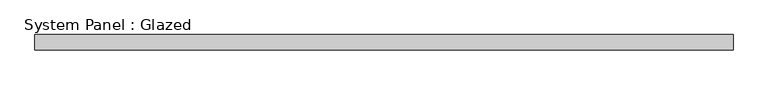
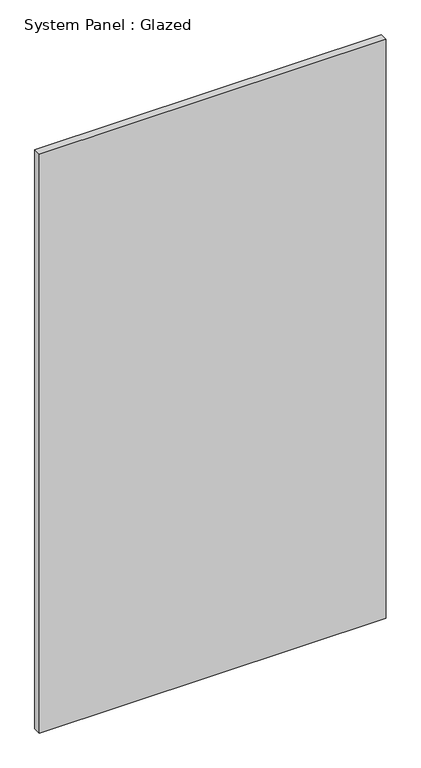
"""IFC4 building model written with IfcOpenShell, lengths in millimetres: plate geometry, System Panel : Glazed."""

from ifc_helpers import new_model, si_unit, origin, origin_with_axes, place, context, project, spatial, polyline, outline, extrude, source, transform, mapped, element, save


def system_panel_glazed_55699693(model_context):
    return source(origin(), model_context, "Body", "SweptSolid", [
        extrude(outline(polyline([(577.85, 19.05), (-577.85, 19.05), (-577.85, 44.45), (577.85, 44.45), (577.85, 19.05)])), origin_with_axes(), (0.0, 0.0, 1.0), 2038.35),
    ])


if __name__ == "__main__":
    model = new_model("IFC4")
    model_context = context("Model", 3, world=origin())
    ifc_project = project(units=[si_unit("LENGTHUNIT", "METRE", prefix="MILLI")], contexts=[model_context])
    site = spatial("IfcSite", under=ifc_project)
    building = spatial("IfcBuilding", under=site)
    placement = place(None, origin())
    system_panel_glazed_shape = system_panel_glazed_55699693(model_context)
    element("IfcPlate", 1, ObjectType="System Panel : Glazed", at=placement, inside=building, context=model_context, shape_type="MappedRepresentation", body=[
        mapped(system_panel_glazed_shape, transform((0.0, 0.0, 0.0), x_axis=(1.0, 0.0, 0.0), y_axis=(0.0, 1.0, 0.0), z_axis=(0.0, 0.0, 1.0))),
    ])
    save(model, "model.ifc")

# Revit data of these elements
# Type "System Panel : Glazed"
#   Construction Type Id = "GSP4R"
#   Analytic Construction = "1/8 in Pilkington single glazing"
#   Visual Light Transmittance = 0.9
#   Solar Heat Gain Coefficient = 0.86
#   Heat Transfer Coefficient (U) = 1.18115 BTU/(h·ft²·°F)
#   Define Thermal Properties by = 1
# Element 1 (IfcPlate, "System Panel : Glazed")
#   Materials on its faces: "Glass"
# Materials
#   "Glass": class "Glass", colour RGB 0 128 192, transparency 0.75, Description = "Soda Lime Glass", Cost = 0
